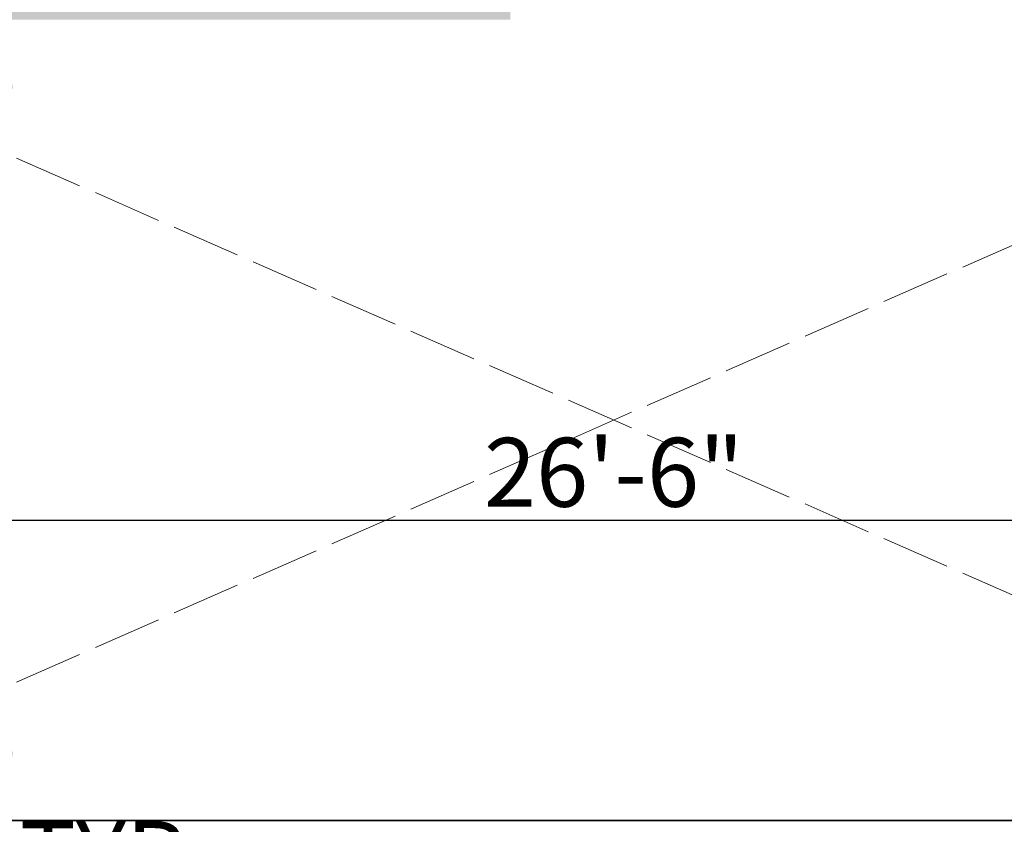
# Model space of a CAD drawing. Units: inches. Extents: x 2083 to 3317, y 1141 to 2115.
# Tile 107 of 256: x 2600 to 2772, y 1272 to 1412. Entities that reach past the tile are written whole.
import ezdxf

# ---------------------------------------------------------------- set-up
doc = ezdxf.new("R2010")
doc.units = ezdxf.units.IN
doc.linetypes.add('ACAD_ISO02W100', pattern=[15, 12, -3])
for name, color, linetype, lineweight in [('A-ANNO-DIMS', 2, 'Continuous', 18), ('A-FLOR-OPEN', 8, 'ACAD_ISO02W100', 13), ('A-WALL', 7, 'Continuous', 35)]:
    doc.layers.add(name, color=color, linetype=linetype, lineweight=lineweight)
doc.layers.add('A-WALL-PATT', color=251, linetype='Continuous', lineweight=13, true_color=0x636466)
doc.styles.get("Standard").update_dxf_attribs({"font": 'arial.ttf'})
doc.dimstyles.new('ISO-25', dxfattribs={"dimtxt": 12, "dimasz": 12, "dimexe": 1.25, "dimexo": 0.625, "dimtad": 1, "dimlunit": 3, "dimtxsty": 'Standard', "dimcen": 2.5, "dimadec": 0, "dimazin": 0, "dimtfac": 1, "dimtmove": 0, "dimatfit": 3, "dimfxl": 1, "dimarcsym": 0})

# ---------------------------------------------------------------- blocks, each defined once
blk = doc.blocks.new('*D25')
at = {"layer": 'A-ANNO-DIMS', "color": 0, "lineweight": -2, "transparency": 16777216}
for p, q in [((2511.96, 1271.64), (2511.96, 1256.61)), ((2535.96, 1271.64), (2535.96, 1256.61)), ((2499.96, 1257.86), (2487.96, 1257.86)), ((2511.96, 1257.86), (2535.96, 1257.86)), ((2547.96, 1257.86), (2634.56, 1257.86))]:
    blk.add_line(p, q, dxfattribs=at)
at = {"layer": 'A-ANNO-DIMS', "color": 0, "transparency": 16777216}
for points in [[(2499.96, 1259.86), (2499.96, 1255.86), (2511.96, 1257.86)], [(2547.96, 1259.86), (2547.96, 1255.86), (2535.96, 1257.86)]]:
    blk.add_solid(points, dxfattribs=at)
at = {"layer": 'Defpoints', "color": 0, "transparency": 16777216}
for p in [(2511.96, 1272.26), (2535.96, 1272.26), (2535.96, 1257.86)]:
    blk.add_point(p, dxfattribs=at)
at = {"layer": 'A-ANNO-DIMS', "color": 0, "transparency": 16777216, "insert": (2597.26, 1264.61), "char_height": 12, "attachment_point": 5}
blk.add_mtext('2\'-0" TYP.', dxfattribs=at)
blk = doc.blocks.new('*D66')
at = {"layer": 'A-ANNO-DIMS', "color": 0, "lineweight": -2, "transparency": 16777216}
for p, q in [((2544.96, 1272.89), (2544.96, 1325.86)), ((2556.96, 1324.61), (2850.96, 1324.61)), ((2862.96, 1272.89), (2862.96, 1325.86))]:
    blk.add_line(p, q, dxfattribs=at)
at = {"layer": 'A-ANNO-DIMS', "color": 0, "transparency": 16777216}
for points in [[(2556.96, 1326.61), (2556.96, 1322.61), (2544.96, 1324.61)], [(2850.96, 1326.61), (2850.96, 1322.61), (2862.96, 1324.61)]]:
    blk.add_solid(points, dxfattribs=at)
at = {"layer": 'Defpoints', "color": 0, "transparency": 16777216}
for p in [(2862.96, 1324.61), (2544.96, 1272.26), (2862.96, 1272.26)]:
    blk.add_point(p, dxfattribs=at)
at = {"layer": 'A-ANNO-DIMS', "color": 0, "transparency": 16777216, "insert": (2703.96, 1331.36), "char_height": 12, "attachment_point": 5}
blk.add_mtext('26\'-6"', dxfattribs=at)
blk = doc.blocks.new('*D67')
at = {"layer": 'A-ANNO-DIMS', "color": 0, "lineweight": -2, "transparency": 16777216}
for p, q in [((2545.58, 1411.76), (2598.56, 1411.76)), ((2597.31, 1399.76), (2597.31, 1284.26)), ((2545.58, 1272.26), (2598.56, 1272.26))]:
    blk.add_line(p, q, dxfattribs=at)
at = {"layer": 'A-ANNO-DIMS', "color": 0, "transparency": 16777216}
for points in [[(2595.31, 1399.76), (2599.31, 1399.76), (2597.31, 1411.76)], [(2595.31, 1284.26), (2599.31, 1284.26), (2597.31, 1272.26)]]:
    blk.add_solid(points, dxfattribs=at)
at = {"layer": 'Defpoints', "color": 0, "transparency": 16777216}
for p in [(2544.96, 1411.76), (2544.96, 1272.26), (2597.31, 1272.26)]:
    blk.add_point(p, dxfattribs=at)
at = {"layer": 'A-ANNO-DIMS', "color": 0, "transparency": 16777216, "insert": (2590.48, 1342.01), "char_height": 12, "attachment_point": 5, "rotation": 90}
blk.add_mtext('11\'-7 1/2"', dxfattribs=at)

msp = doc.modelspace()

# ---------------------------------------------------------------- hatches: boundary and pattern name
at = {"layer": 'A-WALL-PATT'}
h = msp.add_hatch(color=256, dxfattribs=at)
h.dxf.hatch_style = 1
h.paths.add_polyline_path([(3126.96, 2020.761), (2748.96, 2020.761), (2604.96, 2020.761), (2226.96, 2020.761), (2226.96, 1702.761), (2466.96, 1702.761), (2466.96, 1582.761), (2418.96, 1582.761), (2418.96, 1477.761), (2226.96, 1477.761), (2226.96, 1263.261), (2544.96, 1263.261), (2544.96, 1411.761), (2604.96, 1411.761), (2685.96, 1411.761), (2685.96, 1420.761), (2604.96, 1420.761), (2604.96, 1573.761), (2604.96, 1702.761), (2604.96, 2011.761), (2748.96, 2011.761), (2748.96, 1702.761), (2862.96, 1702.761), (2862.96, 1621.761), (2871.96, 1621.761), (2871.96, 1702.761), (2883.96, 1702.761), (2883.96, 1706.939, -0.0264593), (2883.96, 1711.761), (2757.96, 1711.761), (2757.96, 1807.761), (2787.96, 1807.761), (2787.96, 1812.261), (2757.96, 1812.261), (2757.96, 2011.761), (2877.96, 2011.761), (2877.96, 1812.261), (2847.96, 1812.261), (2847.96, 1807.761), (2889.836, 1807.761), (2889.836, 1812.261), (2882.46, 1812.261), (2882.46, 2011.761), (3117.96, 2011.761), (3117.96, 1812.261), (2937.836, 1812.261), (2937.836, 1807.761), (2995.71, 1807.761), (2995.71, 1796.118), (3000.21, 1796.118), (3000.21, 1807.761), (3117.96, 1807.761), (3117.96, 1711.761), (3000.21, 1711.761), (3000.21, 1760.118), (2998.573, 1760.118, -0.020711), (2995.71, 1760.118), (2995.71, 1711.761), (2931.96, 1711.761), (2931.96, 1702.761), (3126.96, 1702.761)])
h.paths.add_polyline_path([(2471.46, 2011.761), (2471.46, 1810.011), (2462.717, 1810.011), (2462.717, 1805.511), (2505.96, 1805.511), (2505.96, 1810.011), (2475.96, 1810.011), (2475.96, 2011.761), (2595.96, 2011.761), (2595.96, 1810.011), (2565.96, 1810.011), (2565.96, 1805.511), (2595.96, 1805.511), (2595.96, 1711.761), (2235.96, 1711.761), (2235.96, 1805.511), (2353.71, 1805.511), (2353.71, 1796.054), (2358.21, 1796.054), (2358.21, 1805.511), (2414.717, 1805.511), (2414.717, 1810.011), (2235.96, 1810.011), (2235.96, 2011.761)], flags=16)
h.paths.add_polyline_path([(2270.205, 1994.61), (2270.205, 1970.61), (2246.205, 1970.61), (2246.205, 1994.61)], flags=0)
edge = h.paths.add_edge_path(flags=0)
edge.add_ellipse((2332.027, 1899.798), major_axis=(-3.043, 3.043), ratio=0.1682525, start_angle=-161.33217, end_angle=-156.30711, ccw=False)
edge.add_ellipse((2333.082, 1898.744), major_axis=(-1.055, 1.055), ratio=0.4535321, start_angle=-123.37102, end_angle=-94.15911)
edge = h.paths.add_edge_path(flags=0)
edge.add_ellipse((2332.027, 1968.876), major_axis=(3.043, 3.043), ratio=0.1682525, start_angle=18.66783, end_angle=23.69289)
edge.add_spline(control_points=[(2332.926, 1970.691), (2332.227, 1970.336), (2330.894, 1969.659), (2328.413, 1970.932), (2327.204, 1967.749), (2324.71, 1969.956), (2322.533, 1967.012), (2320.013, 1971.296), (2317.68, 1968.158), (2316.041, 1967.102), (2315.427, 1966.81)], knot_values=[0, 0, 0, 0, 2.2670587, 4.3245589, 6.6855835, 8.8786411, 11.121502, 14.300359, 17.7552837, 19.732645, 19.732645, 19.732645, 19.732645], degree=3, periodic=0)
edge.add_ellipse((2332.027, 1968.876), major_axis=(3.043, 3.043), ratio=0.1682525, start_angle=18.66783, end_angle=23.69289, ccw=False)
edge.add_ellipse((2333.082, 1969.931), major_axis=(1.055, 1.055), ratio=0.4535321, start_angle=56.62898, end_angle=85.84089, ccw=False)
edge = h.paths.add_edge_path(flags=0)
edge.add_spline(control_points=[(2296.428, 1967.988), (2293.628, 1965.336), (2287.704, 1959.727), (2299.744, 1949.996), (2294.533, 1935.669), (2290.573, 1920.604), (2293.394, 1909.974), (2296.185, 1904.967)], knot_values=[0.0991853, 0.0991853, 0.0991853, 0.0991853, 0.3453009, 0.6198217, 0.9826526, 1.3860932, 1.8105546, 1.8105546, 1.8105546, 1.8105546], degree=3, periodic=0)
edge.add_spline(control_points=[(2296.185, 1904.967), (2297.384, 1902.619), (2298.001, 1901.949), (2298.553, 1901.468)], knot_values=[0.0062457, 0.0062457, 0.0062457, 0.0062457, 0.0554759, 0.0554759, 0.0554759, 0.0554759], degree=3, periodic=0)
edge.add_spline(control_points=[(2298.553, 1901.468), (2297.259, 1900.923), (2295.225, 1900.232), (2293.06, 1900.614), (2292.101, 1900.788), (2292.09, 1900.791)], knot_values=[0.3128349, 0.3128349, 0.3128349, 0.3128349, 0.4017797, 0.4749867, 0.4759027, 0.4759027, 0.4759027, 0.4759027], degree=3, periodic=0)
edge.add_arc((2292.794, 1904.664), 3.937, 215.4209, 259.69818, ccw=False)
edge.add_spline(control_points=[(2289.585, 1902.382), (2289.477, 1902.535), (2289.368, 1902.688), (2289.261, 1902.841)], knot_values=[0.1028719, 0.1028719, 0.1028719, 0.1028719, 0.1168958, 0.1168958, 0.1168958, 0.1168958], degree=3, periodic=0)
edge.add_spline(control_points=[(2289.261, 1902.841), (2288.687, 1902.55), (2287.64, 1902.02), (2285.881, 1901.874), (2283.853, 1901.504), (2281.72, 1899.711), (2278.467, 1899.493), (2276.157, 1901.883), (2272.259, 1899.804), (2267.778, 1901.843), (2262.244, 1900.184), (2257.415, 1901.782), (2254.318, 1900.726), (2253.178, 1900.337)], knot_values=[0, 0, 0, 0, 1.9079767, 3.4771759, 5.261074, 7.9728515, 11.6802485, 13.7179214, 16.9395917, 22.789562, 27.5025027, 33.5952153, 37.1456181, 37.1456181, 37.1456181, 37.1456181], degree=3, periodic=0)
edge.add_line((2253.178, 1900.337), (2250.244, 1902.841))
edge.add_line((2250.244, 1902.841), (2250.244, 1965.833))
edge.add_line((2250.244, 1965.833), (2253.178, 1968.337))
edge.add_spline(control_points=[(2253.178, 1968.337), (2254.318, 1967.948), (2257.415, 1966.892), (2262.244, 1968.49), (2267.778, 1966.831), (2271.527, 1968.537), (2273.876, 1967.828), (2274.207, 1967.728)], knot_values=[0, 0, 0, 0, 0.0901802, 0.2449351, 0.3646438, 0.5132331, 0.5378548, 0.5378548, 0.5378548, 0.5378548], degree=3, periodic=0)
edge.add_arc((2274.353, 1963.793), 3.937, 72.05113, 92.12795, ccw=False)
edge.add_arc((2281.297, 1985.23), 18.596, 252.05113, 288.56572)
edge.add_arc((2292.317, 1956.029), 12.646, 71.02679, 113.77822, ccw=False)
edge = h.paths.add_edge_path(flags=0)
edge.add_spline(control_points=[(2274.899, 1951.856), (2275.066, 1951.617), (2275.233, 1951.377), (2275.398, 1951.136)], knot_values=[1.4099157, 1.4099157, 1.4099157, 1.4099157, 1.4315903, 1.4315903, 1.4315903, 1.4315903], degree=3, periodic=0)
edge.add_spline(control_points=[(2275.398, 1951.136), (2275.792, 1950.562), (2276.179, 1949.984), (2276.546, 1949.397)], knot_values=[1.3582378, 1.3582378, 1.3582378, 1.3582378, 1.4099157, 1.4099157, 1.4099157, 1.4099157], degree=3, periodic=0)
edge.add_line((2276.546, 1949.397), (2277.437, 1947.862))
edge.add_spline(control_points=[(2277.437, 1947.862), (2276.304, 1945.673), (2274.64, 1942.427), (2274.632, 1938.094), (2272.799, 1930.852), (2274.356, 1943.897), (2275.948, 1947.923), (2276.546, 1949.397)], knot_values=[0.0056315, 0.0056315, 0.0056315, 0.0056315, 0.1860139, 0.2660015, 0.3570872, 0.5963902, 0.7397317, 0.7397317, 0.7397317, 0.7397317], degree=3, periodic=0)
edge.add_spline(control_points=[(2276.546, 1949.397), (2276.179, 1949.984), (2275.792, 1950.562), (2275.398, 1951.136)], knot_values=[1.3582378, 1.3582378, 1.3582378, 1.3582378, 1.4099157, 1.4099157, 1.4099157, 1.4099157], degree=3, periodic=0)
edge.add_spline(control_points=[(2275.398, 1951.136), (2274.943, 1950.08), (2274.208, 1948.025), (2273.935, 1944.851), (2272.469, 1937.627), (2273.466, 1945.696), (2274.701, 1951.059), (2274.899, 1951.856)], knot_values=[0.1043639, 0.1043639, 0.1043639, 0.1043639, 0.1896363, 0.2696239, 0.3607096, 0.6000126, 0.6446217, 0.6446217, 0.6446217, 0.6446217], degree=3, periodic=0)
h.paths.add_polyline_path([(2269.168, 1963.128, -0.3575267), (2268.171, 1960.976, -0.0925607), (2268.171, 1939.436, -0.3575267), (2269.168, 1937.285, -0.3575267), (2267.016, 1938.282, -0.1647847), (2254.686, 1938.282, -0.3575267), (2252.534, 1937.285, -0.3575267), (2253.531, 1939.436, -0.0925607), (2253.531, 1960.976, -0.3575267), (2252.534, 1963.128, -0.3575267), (2254.686, 1962.131, -0.1647847), (2267.016, 1962.131, -0.3575267)], flags=0)
h.paths.add_polyline_path([(2248.874, 1967.802), (2248.874, 1957.028), (2249.458, 1957.028), (2249.458, 1911.647), (2248.874, 1911.647), (2248.874, 1900.873), (2246.512, 1900.873, 0.1973271), (2244.15, 1902.457), (2244.15, 1966.218, 0.1973271), (2246.512, 1967.802)], flags=0)
h.paths.add_polyline_path([(2269.168, 1931.389, -0.3575267), (2268.171, 1929.238, -0.0925607), (2268.171, 1907.698, -0.3575267), (2269.168, 1905.547, -0.3575267), (2267.016, 1906.544, -0.1647847), (2254.686, 1906.544, -0.3575267), (2252.534, 1905.547, -0.3575267), (2253.531, 1907.698, -0.0925607), (2253.531, 1929.238, -0.3575267), (2252.534, 1931.389, -0.3575267), (2254.686, 1930.392, -0.1647847), (2267.016, 1930.392, -0.3575267)], flags=0)
edge = h.paths.add_edge_path(flags=0)
edge.add_spline(control_points=[(2276.197, 1906.724), (2276.168, 1909.029), (2276.114, 1913.372), (2270.598, 1924.925), (2273.905, 1919.013), (2275.922, 1916.262), (2275.475, 1912.402), (2277.258, 1910.381), (2276.696, 1908.225), (2276.646, 1906.813), (2276.618, 1906.008)], knot_values=[0, 0, 0, 0, 8.6102597, 16.2212739, 18.8430575, 23.8048978, 27.4408283, 29.3561016, 31.2034776, 33.6506866, 33.6506866, 33.6506866, 33.6506866], degree=3, periodic=0)
edge.add_spline(control_points=[(2276.618, 1906.008), (2276.623, 1905.624), (2276.498, 1904.629), (2275.442, 1903.855), (2274.937, 1903.08), (2274.859, 1902.841)], knot_values=[0.1564884, 0.1564884, 0.1564884, 0.1564884, 0.1843975, 0.2313765, 0.2505985, 0.2505985, 0.2505985, 0.2505985], degree=3, periodic=0)
edge.add_line((2274.859, 1902.841), (2276.506, 1902.841))
edge.add_spline(control_points=[(2276.506, 1902.841), (2276.788, 1903.085), (2277.665, 1904.125), (2278.25, 1904.341), (2277.654, 1908.527), (2278.156, 1906.228), (2278.1, 1905.286), (2278.847, 1904.069), (2277.857, 1903.415), (2277.874, 1902.991), (2277.904, 1902.841)], knot_values=[0.0595743, 0.0595743, 0.0595743, 0.0595743, 0.0807529, 0.1037415, 0.1697201, 0.1760361, 0.2071372, 0.2404744, 0.2623409, 0.2736605, 0.2736605, 0.2736605, 0.2736605], degree=3, periodic=0)
edge.add_line((2277.904, 1902.841), (2280.03, 1902.841))
edge.add_spline(control_points=[(2280.03, 1902.841), (2279.888, 1903.088), (2279.499, 1903.982), (2280.152, 1905.939), (2278.104, 1909.658), (2279.762, 1907.185), (2280.328, 1904.875), (2280.485, 1903.49), (2281.463, 1903.249), (2281.758, 1902.936), (2281.834, 1902.841)], knot_values=[0.013856, 0.013856, 0.013856, 0.013856, 0.0348738, 0.0888667, 0.1078792, 0.1267378, 0.158714, 0.1937575, 0.2174868, 0.2267221, 0.2267221, 0.2267221, 0.2267221], degree=3, periodic=0)
edge.add_spline(control_points=[(2281.834, 1902.841), (2281.788, 1902.827), (2281.647, 1902.783), (2281.396, 1902.859), (2281.088, 1902.985), (2280.721, 1903.061), (2280.333, 1903.026), (2280.125, 1902.899), (2280.03, 1902.841)], knot_values=[0, 0, 0, 0, 0.1441304, 0.435517, 0.7492759, 1.1530457, 1.5483707, 1.878348, 1.878348, 1.878348, 1.878348], degree=3, periodic=0)
edge.add_line((2280.03, 1902.841), (2277.904, 1902.841))
edge.add_spline(control_points=[(2277.904, 1902.841), (2277.893, 1902.796), (2277.865, 1902.68), (2277.607, 1902.687), (2277.274, 1902.801), (2276.838, 1902.62), (2276.584, 1902.789), (2276.506, 1902.841)], knot_values=[0, 0, 0, 0, 0.1271885, 0.3261988, 0.6280094, 1.2435704, 1.5153306, 1.5153306, 1.5153306, 1.5153306], degree=3, periodic=0)
edge.add_line((2276.506, 1902.841), (2274.859, 1902.841))
edge.add_spline(control_points=[(2274.859, 1902.841), (2274.814, 1902.899), (2274.725, 1903.013), (2274.493, 1903.119), (2274.244, 1902.961), (2273.937, 1903.185), (2273.614, 1902.983), (2273.408, 1902.883), (2273.322, 1902.841)], knot_values=[0, 0, 0, 0, 0.2184302, 0.4369566, 0.6879766, 0.9903786, 1.3983955, 1.6918498, 1.6918498, 1.6918498, 1.6918498], degree=3, periodic=0)
edge.add_spline(control_points=[(2273.322, 1902.841), (2273.617, 1903.446), (2274.274, 1904.538), (2276.027, 1904.574), (2276.207, 1906.584), (2276.197, 1906.724)], knot_values=[0.0122268, 0.0122268, 0.0122268, 0.0122268, 0.0594721, 0.1062177, 0.134458, 0.134458, 0.134458, 0.134458], degree=3, periodic=0)
h.paths.add_polyline_path([(2270.776, 1897.79), (2270.776, 1873.79), (2246.776, 1873.79), (2246.776, 1897.79)], flags=0)
h.paths.add_polyline_path([(2353.71, 1760.005), (2353.71, 1760.054), (2358.21, 1760.054, -0.033729)], flags=0)
h.paths.add_polyline_path([(2321.819, 1737.529), (2341.995, 1737.529, -0.4142136), (2343.203, 1736.321), (2343.203, 1721.021, -0.4142136), (2341.995, 1719.813), (2321.819, 1719.813, -0.4142136), (2320.611, 1721.021), (2320.611, 1736.321, -0.4142136)], flags=0)
h.paths.add_polyline_path([(2324.235, 1736.321), (2339.579, 1736.321, -0.4142136), (2341.995, 1733.905), (2341.995, 1725.45, -0.4142136), (2339.579, 1723.034), (2333.681, 1723.034), (2333.845, 1722.045, -0.8706461), (2335.425, 1721.826, -0.767327), (2333.923, 1721.423), (2331.291, 1721.423, -0.767327), (2329.788, 1721.826, -0.8706461), (2331.368, 1722.045), (2331.533, 1723.034), (2324.235, 1723.034, -0.4142136), (2321.819, 1725.45), (2321.819, 1733.905, -0.4142136)], flags=0)
h.paths.add_polyline_path([(2570.484, 1928.615), (2589.684, 1928.615), (2590.169, 1928.615), (2590.169, 1904.993), (2570.484, 1904.993)], flags=0)
h.paths.add_polyline_path([(2574.447, 1927.264, -1), (2572.829, 1927.264, -1)], flags=0)
h.paths.add_polyline_path([(2573.09, 1926.941), (2573.925, 1927.776), (2574.148, 1927.553), (2573.313, 1926.718)], flags=0)
h.paths.add_polyline_path([(2578.779, 1919.73, -1), (2571.592, 1919.73, -1)], flags=0)
h.paths.add_polyline_path([(2578.385, 1919.73, -1), (2571.985, 1919.73, -1)], flags=0)
h.paths.add_polyline_path([(2331.596, 1729.476, -1), (2333.618, 1729.476, -1)], flags=0)
h.paths.add_polyline_path([(2578.034, 1927.264, -1), (2576.416, 1927.264, -1)], flags=0)
h.paths.add_polyline_path([(2576.689, 1927.531), (2576.912, 1927.754), (2577.747, 1926.919), (2577.524, 1926.696)], flags=0)
h.paths.add_polyline_path([(2578.139, 1909.86, -1), (2572.232, 1909.86, -1)], flags=0)
h.paths.add_polyline_path([(2577.745, 1909.86, -1), (2572.625, 1909.86, -1)], flags=0)
h.paths.add_polyline_path([(2583.798, 1927.264, -1), (2582.179, 1927.264, -1)], flags=0)
h.paths.add_polyline_path([(2582.719, 1927.754), (2583.554, 1926.919), (2583.331, 1926.696), (2582.496, 1927.531)], flags=0)
h.paths.add_polyline_path([(2582.496, 1927.531), (2582.719, 1927.754), (2583.554, 1926.919), (2583.331, 1926.696)], flags=0)
h.paths.add_polyline_path([(2587.739, 1920.53, -1), (2581.832, 1920.53, -1)], flags=0)
h.paths.add_polyline_path([(2587.345, 1920.53, -1), (2582.225, 1920.53, -1)], flags=0)
h.paths.add_polyline_path([(2587.385, 1927.264, -1), (2585.766, 1927.264, -1)], flags=0)
h.paths.add_polyline_path([(2586.082, 1926.98), (2586.917, 1927.815), (2587.14, 1927.593), (2586.305, 1926.758)], flags=0)
h.paths.add_polyline_path([(2588.379, 1910.66, -1), (2581.192, 1910.66, -1)], flags=0)
h.paths.add_polyline_path([(2587.985, 1910.66, -1), (2581.585, 1910.66, -1)], flags=0)
h.paths.add_polyline_path([(2417.168, 1729.478), (2437.344, 1729.478, -0.4142136), (2438.552, 1728.27), (2438.552, 1712.969, -0.4142136), (2437.344, 1711.761), (2417.168, 1711.761, -0.4142136), (2415.96, 1712.969), (2415.96, 1728.27, -0.4142136)], flags=0)
h.paths.add_polyline_path([(2419.584, 1728.27), (2434.928, 1728.27, -0.4142136), (2437.344, 1725.854), (2437.344, 1717.398, -0.4142136), (2434.928, 1714.983), (2429.029, 1714.983), (2429.194, 1713.994, -0.8706461), (2430.774, 1713.775, -0.767327), (2429.271, 1713.372), (2426.64, 1713.372, -0.767327), (2425.137, 1713.775, -0.8706461), (2426.717, 1713.994), (2426.882, 1714.983), (2419.584, 1714.983, -0.4142136), (2417.168, 1717.398), (2417.168, 1725.854, -0.4142136)], flags=0)
h.paths.add_polyline_path([(2419.584, 1728.27), (2434.928, 1728.27, -0.4142136), (2437.344, 1725.854), (2437.344, 1717.398, -0.4142136), (2434.928, 1714.983), (2429.029, 1714.983), (2428.358, 1719.009), (2427.553, 1719.009), (2426.882, 1714.983), (2419.584, 1714.983, -0.4142136), (2417.168, 1717.398), (2417.168, 1725.854, -0.4142136)], flags=0)
h.paths.add_polyline_path([(2426.944, 1721.425, -1), (2428.967, 1721.425, -1)], flags=0)
h.paths.add_polyline_path([(2475.96, 1702.761), (2595.96, 1702.761), (2595.96, 1582.761), (2475.96, 1582.761)], flags=16)
h.paths.add_polyline_path([(2427.96, 1573.761), (2595.96, 1573.761), (2595.96, 1468.761), (2595.96, 1420.761), (2384.46, 1420.761), (2384.46, 1468.761), (2427.96, 1468.761)], flags=16)
h.paths.add_polyline_path([(2379.96, 1468.761), (2379.96, 1420.761), (2235.96, 1420.761), (2235.96, 1468.761)], flags=16)
h.paths.add_polyline_path([(2317.816, 1466.696), (2337.992, 1466.696, -0.4142136), (2339.2, 1465.488), (2339.2, 1450.187, -0.4142136), (2337.992, 1448.979), (2317.816, 1448.979, -0.4142136), (2316.608, 1450.187), (2316.608, 1465.488, -0.4142136)], flags=0)
h.paths.add_polyline_path([(2320.232, 1465.488), (2335.576, 1465.488, -0.4142136), (2337.992, 1463.072), (2337.992, 1454.616, -0.4142136), (2335.576, 1452.2), (2329.677, 1452.2), (2329.842, 1451.212, -0.8706461), (2331.422, 1450.992, -0.767327), (2329.92, 1450.59), (2327.288, 1450.59, -0.767327), (2325.785, 1450.992, -0.8706461), (2327.365, 1451.212), (2327.53, 1452.2), (2320.232, 1452.2, -0.4142136), (2317.816, 1454.616), (2317.816, 1463.072, -0.4142136)], flags=0)
h.paths.add_polyline_path([(2320.232, 1465.488), (2335.576, 1465.488, -0.4142136), (2337.992, 1463.072), (2337.992, 1454.616, -0.4142136), (2335.576, 1452.2), (2329.677, 1452.2), (2329.006, 1456.227), (2328.201, 1456.227), (2327.53, 1452.2), (2320.232, 1452.2, -0.4142136), (2317.816, 1454.616), (2317.816, 1463.072, -0.4142136)], flags=0)
h.paths.add_polyline_path([(2327.593, 1458.643, -1), (2329.615, 1458.643, -1)], flags=0)
h.paths.add_polyline_path([(2244.412, 1433.34), (2241.921, 1433.34, -0.4142136), (2240.018, 1435.244), (2240.018, 1440.953, -0.4142105), (2241.921, 1442.856), (2244.412, 1442.856, -1.9764724)], flags=0)
h.paths.add_polyline_path([(2245.357, 1434.398, -0.4142136), (2245.357, 1441.799, -2.1440985)], flags=0)
h.paths.add_polyline_path([(2535.96, 1416.261), (2535.96, 1272.261), (2235.96, 1272.261), (2235.96, 1416.261)], flags=16)
h.paths.add_polyline_path([(2260.12, 1384.293), (2260.12, 1362.039), (2237.865, 1362.039), (2237.865, 1384.293)], flags=0)
edge = h.paths.add_edge_path(flags=0)
edge.add_line((2318.252, 1362.093), (2318.146, 1362.001))
edge.add_ellipse((2317.445, 1360.431), major_axis=(2.822, 2.822), ratio=0.1682525, start_angle=18.66783, end_angle=20.94813, ccw=False)
edge.add_ellipse((2318.423, 1361.409), major_axis=(0.978, 0.978), ratio=0.4535321, start_angle=56.62898, end_angle=70.2262, ccw=False)
edge = h.paths.add_edge_path(flags=0)
edge.add_line((2319.107, 1295.571), (2319.015, 1295.677))
edge.add_ellipse((2317.445, 1296.378), major_axis=(-2.822, 2.822), ratio=0.1682525, start_angle=-161.33217, end_angle=-159.05187, ccw=False)
edge.add_ellipse((2318.423, 1295.4), major_axis=(-0.978, 0.978), ratio=0.4535321, start_angle=-123.37102, end_angle=-109.7738)
edge = h.paths.add_edge_path(flags=0)
edge.add_spline(control_points=[(2284.21, 1301.17), (2284.581, 1300.445), (2284.891, 1299.892), (2285.16, 1299.461)], knot_values=[0.0390658, 0.0390658, 0.0390658, 0.0390658, 0.0554759, 0.0554759, 0.0554759, 0.0554759], degree=3, periodic=0)
edge.add_line((2285.16, 1299.461), (2284.21, 1301.17))
edge = h.paths.add_edge_path(flags=0)
edge.add_line((2280.412, 1297.298), (2283.37, 1297.036))
edge.add_line((2283.37, 1297.036), (2286.406, 1297.926))
edge.add_spline(control_points=[(2286.406, 1297.926), (2285.305, 1297.463), (2284.345, 1297.129), (2283.37, 1297.036)], knot_values=[0.3943688, 0.3943688, 0.3943688, 0.3943688, 0.4759027, 0.4759027, 0.4759027, 0.4759027], degree=3, periodic=0)
edge.add_spline(control_points=[(2283.37, 1297.036), (2283.281, 1297.028), (2282.316, 1296.957), (2281.313, 1297.134), (2280.423, 1297.296), (2280.412, 1297.298)], knot_values=[0.3128349, 0.3128349, 0.3128349, 0.3128349, 0.3202458, 0.3934528, 0.3943688, 0.3943688, 0.3943688, 0.3943688], degree=3, periodic=0)
edge = h.paths.add_edge_path(flags=0)
edge.add_line((2284.436, 1359.607), (2280.446, 1355.328))
edge.add_line((2280.446, 1355.328), (2279.58, 1351.018))
edge.add_line((2279.58, 1351.018), (2282.413, 1346.58))
edge.add_spline(control_points=[(2282.413, 1346.58), (2283.153, 1345.589), (2284.253, 1344.029), (2284.801, 1342.387), (2284.935, 1341.806)], knot_values=[1.2400982, 1.2400982, 1.2400982, 1.2400982, 1.3328922, 1.3827123, 1.3827123, 1.3827123, 1.3827123], degree=3, periodic=0)
edge.add_spline(control_points=[(2284.935, 1341.806), (2285.319, 1340.141), (2285.233, 1338.409), (2284.91, 1336.654)], knot_values=[1.0974841, 1.0974841, 1.0974841, 1.0974841, 1.2400982, 1.2400982, 1.2400982, 1.2400982], degree=3, periodic=0)
edge.add_spline(control_points=[(2284.91, 1336.654), (2284.587, 1334.899), (2284.027, 1333.12), (2283.463, 1331.361)], knot_values=[0.9548699, 0.9548699, 0.9548699, 0.9548699, 1.0974841, 1.0974841, 1.0974841, 1.0974841], degree=3, periodic=0)
edge.add_line((2283.463, 1331.361), (2281.89, 1326.153))
edge.add_line((2281.89, 1326.153), (2280.756, 1321.056))
edge.add_line((2280.756, 1321.056), (2280.299, 1316.002))
edge.add_line((2280.299, 1316.002), (2280.716, 1310.95))
edge.add_line((2280.716, 1310.95), (2282.028, 1305.972))
edge.add_line((2282.028, 1305.972), (2284.21, 1301.17))
edge.add_spline(control_points=[(2284.21, 1301.17), (2283.341, 1302.73), (2282.612, 1304.336), (2282.028, 1305.972)], knot_values=[0.0991853, 0.0991853, 0.0991853, 0.0991853, 0.2417994, 0.2417994, 0.2417994, 0.2417994], degree=3, periodic=0)
edge.add_spline(control_points=[(2282.028, 1305.972), (2281.444, 1307.608), (2281.005, 1309.273), (2280.716, 1310.95)], knot_values=[0.2417994, 0.2417994, 0.2417994, 0.2417994, 0.3844135, 0.3844135, 0.3844135, 0.3844135], degree=3, periodic=0)
edge.add_spline(control_points=[(2280.716, 1310.95), (2280.433, 1312.588), (2280.289, 1314.277), (2280.299, 1315.962), (2280.299, 1316.002)], knot_values=[0.3844135, 0.3844135, 0.3844135, 0.3844135, 0.5236467, 0.5270276, 0.5270276, 0.5270276, 0.5270276], degree=3, periodic=0)
edge.add_spline(control_points=[(2280.299, 1316.002), (2280.312, 1317.687), (2280.478, 1319.368), (2280.756, 1321.056)], knot_values=[0.5270276, 0.5270276, 0.5270276, 0.5270276, 0.6696417, 0.6696417, 0.6696417, 0.6696417], degree=3, periodic=0)
edge.add_spline(control_points=[(2280.756, 1321.056), (2281.035, 1322.744), (2281.426, 1324.44), (2281.89, 1326.153)], knot_values=[0.6696417, 0.6696417, 0.6696417, 0.6696417, 0.8122558, 0.8122558, 0.8122558, 0.8122558], degree=3, periodic=0)
edge.add_spline(control_points=[(2281.89, 1326.153), (2282.264, 1327.533), (2282.788, 1329.262), (2283.353, 1331.018), (2283.463, 1331.361)], knot_values=[0.8122558, 0.8122558, 0.8122558, 0.8122558, 0.9270873, 0.9548699, 0.9548699, 0.9548699, 0.9548699], degree=3, periodic=0)
edge.add_line((2283.463, 1331.361), (2284.91, 1336.654))
edge.add_line((2284.91, 1336.654), (2284.935, 1341.806))
edge.add_line((2284.935, 1341.806), (2282.413, 1346.58))
edge.add_spline(control_points=[(2282.413, 1346.58), (2281.275, 1348.104), (2280.078, 1349.57), (2279.58, 1351.018)], knot_values=[1.3827123, 1.3827123, 1.3827123, 1.3827123, 1.5253264, 1.5253264, 1.5253264, 1.5253264], degree=3, periodic=0)
edge.add_spline(control_points=[(2279.58, 1351.018), (2279.443, 1351.415), (2279.136, 1352.857), (2279.735, 1354.29), (2280.446, 1355.328)], knot_values=[1.5253264, 1.5253264, 1.5253264, 1.5253264, 1.564439, 1.6679405, 1.6679405, 1.6679405, 1.6679405], degree=3, periodic=0)
edge.add_spline(control_points=[(2280.446, 1355.328), (2281.426, 1356.758), (2282.931, 1358.183), (2284.436, 1359.607)], knot_values=[1.6679405, 1.6679405, 1.6679405, 1.6679405, 1.8105546, 1.8105546, 1.8105546, 1.8105546], degree=3, periodic=0)
edge.add_arc((2280.623, 1348.518), 11.726, 71.02679, 113.77822)
edge.add_arc((2270.405, 1375.595), 17.244, 252.05113, 288.56572, ccw=False)
edge.add_arc((2263.966, 1355.718), 3.651, 72.05113, 92.12795)
edge.add_arc((2263.966, 1355.718), 3.651, 92.12795, 177.98513)
edge.add_spline(control_points=[(2260.318, 1355.846), (2260.26, 1354.221), (2260.551, 1350.187), (2262.999, 1346.766), (2264.473, 1344.649)], knot_values=[1.4315903, 1.4315903, 1.4315903, 1.4315903, 1.5641438, 1.7706953, 1.7706953, 1.7706953, 1.7706953], degree=3, periodic=0)
edge.add_line((2264.473, 1344.649), (2264.936, 1343.983))
edge.add_spline(control_points=[(2263.801, 1340.248), (2263.843, 1340.514), (2264.067, 1341.756), (2264.513, 1343.002), (2264.935, 1343.981)], knot_values=[0.5365702, 0.5365702, 0.5365702, 0.5365702, 0.5593494, 0.6446217, 0.6446217, 0.6446217, 0.6446217], degree=3, periodic=0)
edge.add_spline(control_points=[(2264.935, 1343.981), (2265.118, 1343.715), (2265.299, 1343.448), (2265.477, 1343.179)], knot_values=[1.3840767, 1.3840767, 1.3840767, 1.3840767, 1.4099157, 1.4099157, 1.4099157, 1.4099157], degree=3, periodic=0)
edge.add_spline(control_points=[(2265.477, 1343.179), (2265.655, 1342.911), (2265.829, 1342.641), (2265.999, 1342.369)], knot_values=[1.3582378, 1.3582378, 1.3582378, 1.3582378, 1.3840767, 1.3840767, 1.3840767, 1.3840767], degree=3, periodic=0)
edge.add_line((2265.999, 1342.369), (2266.826, 1340.946))
edge.add_spline(control_points=[(2266.826, 1340.946), (2268.894, 1337.09), (2271.398, 1325.843), (2270.516, 1310.569), (2275.919, 1301.861), (2277.79, 1299.199)], knot_values=[0.1168958, 0.1168958, 0.1168958, 0.1168958, 0.4729873, 1.0509689, 1.3137934, 1.3137934, 1.3137934, 1.3137934], degree=3, periodic=0)
edge.add_spline(control_points=[(2277.79, 1299.199), (2277.839, 1299.128), (2277.889, 1299.057), (2277.94, 1298.987)], knot_values=[0.1098839, 0.1098839, 0.1098839, 0.1098839, 0.1168958, 0.1168958, 0.1168958, 0.1168958], degree=3, periodic=0)
edge.add_line((2277.94, 1298.987), (2277.789, 1299.199))
edge.add_spline(control_points=[(2277.789, 1299.199), (2277.257, 1298.929), (2276.286, 1298.438), (2275.039, 1298.334), (2274.383, 1298.239), (2274.215, 1298.209)], knot_values=[33.1218702, 33.1218702, 33.1218702, 33.1218702, 35.0290557, 36.5982549, 37.1448269, 37.1448269, 37.1448269, 37.1448269], degree=3, periodic=0)
edge.add_line((2274.215, 1298.209), (2273.073, 1297.893))
edge.add_spline(control_points=[(2273.073, 1297.893), (2272.323, 1297.58), (2271.039, 1296.511), (2269.248, 1296.226), (2268.423, 1296.375)], knot_values=[26.5325843, 26.5325843, 26.5325843, 26.5325843, 29.198919, 31.8391012, 31.8391012, 31.8391012, 31.8391012], degree=3, periodic=0)
edge.add_line((2268.423, 1296.375), (2263.879, 1297.458))
edge.add_spline(control_points=[(2263.879, 1297.458), (2263.556, 1297.359), (2261.86, 1296.839), (2260.239, 1297.282), (2258.933, 1297.516)], knot_values=[15.9195506, 15.9195506, 15.9195506, 15.9195506, 16.9395917, 21.2260675, 21.2260675, 21.2260675, 21.2260675], degree=3, periodic=0)
edge.add_line((2258.933, 1297.516), (2254.055, 1297.329))
edge.add_spline(control_points=[(2254.055, 1297.329), (2253.756, 1297.296), (2252.114, 1297.165), (2250.462, 1297.544), (2249.13, 1297.668)], knot_values=[5.3065169, 5.3065169, 5.3065169, 5.3065169, 6.2764352, 10.6130337, 10.6130337, 10.6130337, 10.6130337], degree=3, periodic=0)
edge.add_line((2249.13, 1297.668), (2244.332, 1296.878))
edge.add_line((2244.332, 1296.878), (2241.611, 1299.199))
edge.add_line((2241.611, 1299.199), (2241.611, 1357.609))
edge.add_line((2241.611, 1357.609), (2244.332, 1359.931))
edge.add_line((2244.332, 1359.931), (2252.729, 1359.543))
edge.add_spline(control_points=[(2252.729, 1359.543), (2252.871, 1359.546), (2253.306, 1359.548), (2253.74, 1359.514), (2254.032, 1359.482)], knot_values=[0.233291, 0.233291, 0.233291, 0.233291, 0.2449351, 0.2689274, 0.2689274, 0.2689274, 0.2689274], degree=3, periodic=0)
edge.add_line((2254.032, 1359.482), (2259.587, 1359.416))
edge.add_spline(control_points=[(2259.587, 1359.416), (2260.677, 1359.629), (2262.073, 1359.897), (2263.524, 1359.459), (2263.83, 1359.366)], knot_values=[0.4225164, 0.4225164, 0.4225164, 0.4225164, 0.5132331, 0.5378548, 0.5378548, 0.5378548, 0.5378548], degree=3, periodic=0)
edge.add_arc((2263.966, 1355.718), 3.651, 72.05113, 92.12795, ccw=False)
edge.add_arc((2270.405, 1375.595), 17.244, 252.05113, 288.56572)
edge.add_arc((2280.623, 1348.518), 11.726, 71.02679, 113.77822, ccw=False)
h.paths.add_polyline_path([(2240.341, 1359.435), (2240.341, 1349.444), (2240.882, 1349.444), (2240.882, 1307.365), (2240.341, 1307.365), (2240.341, 1297.374), (2238.15, 1297.374, 0.1973271), (2235.96, 1298.843), (2235.96, 1357.966, 0.1973271), (2238.15, 1359.435)], flags=0)
h.paths.add_polyline_path([(2259.158, 1355.101, -0.3575267), (2258.233, 1353.106, -0.0925607), (2258.233, 1333.133, -0.3575267), (2259.158, 1331.138, -0.3575267), (2257.163, 1332.062, -0.1647847), (2245.729, 1332.062, -0.3575267), (2243.735, 1331.138, -0.3575267), (2244.659, 1333.133, -0.0925607), (2244.659, 1353.106, -0.3575267), (2243.735, 1355.101, -0.3575267), (2245.729, 1354.176, -0.1647847), (2257.163, 1354.176, -0.3575267)], flags=0)
edge = h.paths.add_edge_path(flags=0)
edge.add_line((2265.999, 1342.369), (2266.826, 1340.946))
edge.add_line((2266.826, 1340.946), (2265.308, 1337.814))
edge.add_line((2265.308, 1337.814), (2264.358, 1334.653))
edge.add_line((2264.358, 1334.653), (2264.262, 1333.8))
edge.add_spline(control_points=[(2264.262, 1333.8), (2264.208, 1333.187), (2264.162, 1332.366), (2264.007, 1331.414), (2263.969, 1331.202)], knot_values=[0.4644442, 0.4644442, 0.4644442, 0.4644442, 0.5166905, 0.5316081, 0.5316081, 0.5316081, 0.5316081], degree=3, periodic=0)
edge.add_spline(control_points=[(2263.969, 1331.202), (2263.775, 1330.119), (2263.424, 1328.791), (2263.257, 1328.531), (2263.234, 1328.515)], knot_values=[0.3726816, 0.3726816, 0.3726816, 0.3726816, 0.4488497, 0.4644442, 0.4644442, 0.4644442, 0.4644442], degree=3, periodic=0)
edge.add_spline(control_points=[(2263.234, 1328.515), (2263.096, 1328.42), (2263.131, 1329.301), (2263.275, 1330.616)], knot_values=[0.2809191, 0.2809191, 0.2809191, 0.2809191, 0.3726816, 0.3726816, 0.3726816, 0.3726816], degree=3, periodic=0)
edge.add_spline(control_points=[(2263.275, 1330.616), (2263.419, 1331.93), (2263.672, 1333.677), (2263.97, 1335.315)], knot_values=[0.1891566, 0.1891566, 0.1891566, 0.1891566, 0.2809191, 0.2809191, 0.2809191, 0.2809191], degree=3, periodic=0)
edge.add_spline(control_points=[(2263.97, 1335.315), (2264.1, 1336.032), (2264.419, 1337.622), (2264.755, 1338.864), (2264.947, 1339.491)], knot_values=[0.097394, 0.097394, 0.097394, 0.097394, 0.1375775, 0.1891566, 0.1891566, 0.1891566, 0.1891566], degree=3, periodic=0)
edge.add_spline(control_points=[(2264.947, 1339.491), (2265.29, 1340.606), (2265.644, 1341.494), (2265.999, 1342.369)], knot_values=[0.0056315, 0.0056315, 0.0056315, 0.0056315, 0.097394, 0.097394, 0.097394, 0.097394], degree=3, periodic=0)
h.paths.add_polyline_path([(2259.158, 1325.671, -0.3575267), (2258.233, 1323.676, -0.0925607), (2258.233, 1303.703, -0.3575267), (2259.158, 1301.708, -0.3575267), (2257.163, 1302.633, -0.1647847), (2245.729, 1302.633, -0.3575267), (2243.735, 1301.708, -0.3575267), (2244.659, 1303.703, -0.0925607), (2244.659, 1323.676, -0.3575267), (2243.735, 1325.671, -0.3575267), (2245.729, 1324.747, -0.1647847), (2257.163, 1324.747, -0.3575267)], flags=0)
edge = h.paths.add_edge_path(flags=0)
edge.add_spline(control_points=[(2261.709, 1317.311), (2261.679, 1317.418), (2261.762, 1317.389), (2262.491, 1316.09), (2262.962, 1315.301)], knot_values=[14.9558607, 14.9558607, 14.9558607, 14.9558607, 16.2212739, 18.6948259, 18.6948259, 18.6948259, 18.6948259], degree=3, periodic=0)
edge.add_spline(control_points=[(2262.962, 1315.301), (2262.99, 1315.254), (2263.702, 1314.067), (2264.349, 1313.127), (2264.73, 1312.164)], knot_values=[18.6948259, 18.6948259, 18.6948259, 18.6948259, 18.8430575, 22.433791, 22.433791, 22.433791, 22.433791], degree=3, periodic=0)
edge.add_spline(control_points=[(2264.73, 1312.164), (2264.876, 1311.796), (2265.177, 1310.77), (2265.143, 1309.559), (2265.248, 1308.824)], knot_values=[22.433791, 22.433791, 22.433791, 22.433791, 23.8048978, 26.1727562, 26.1727562, 26.1727562, 26.1727562], degree=3, periodic=0)
edge.add_line((2265.248, 1308.824), (2265.851, 1307.172))
edge.add_spline(control_points=[(2265.851, 1307.172), (2266.065, 1306.822), (2266.384, 1306.332), (2266.424, 1305.781), (2266.42, 1305.611)], knot_values=[28.0625624, 28.0625624, 28.0625624, 28.0625624, 29.3561016, 29.9117214, 29.9117214, 29.9117214, 29.9117214], degree=3, periodic=0)
edge.add_spline(control_points=[(2266.42, 1305.611), (2266.416, 1305.433), (2266.394, 1305.25), (2266.365, 1305.066)], knot_values=[29.9117214, 29.9117214, 29.9117214, 29.9117214, 30.4978371, 30.4978371, 30.4978371, 30.4978371], degree=3, periodic=0)
edge.add_line((2266.365, 1305.066), (2266.066, 1302.136))
edge.add_spline(control_points=[(2266.066, 1302.136), (2266.071, 1301.78), (2265.998, 1301.2), (2265.663, 1300.759), (2265.509, 1300.586)], knot_values=[0.1564884, 0.1564884, 0.1564884, 0.1564884, 0.1843975, 0.2035434, 0.2035434, 0.2035434, 0.2035434], degree=3, periodic=0)
edge.add_line((2265.509, 1300.586), (2264.435, 1299.199))
edge.add_line((2264.435, 1299.199), (2265.962, 1299.199))
edge.add_line((2265.962, 1299.199), (2267.336, 1301.175))
edge.add_line((2267.336, 1301.175), (2267.312, 1301.986))
edge.add_spline(control_points=[(2267.312, 1301.986), (2267.261, 1302.862), (2267.16, 1303.737), (2267.271, 1303.326)], knot_values=[0.1262286, 0.1262286, 0.1262286, 0.1262286, 0.1666174, 0.1666174, 0.1666174, 0.1666174], degree=3, periodic=0)
edge.add_spline(control_points=[(2267.271, 1303.326), (2267.28, 1303.294), (2267.31, 1303.175), (2267.373, 1302.884), (2267.406, 1302.683), (2267.418, 1302.601)], knot_values=[0.1666174, 0.1666174, 0.1666174, 0.1666174, 0.1697201, 0.1760361, 0.1807647, 0.1807647, 0.1807647, 0.1807647], degree=3, periodic=0)
edge.add_spline(control_points=[(2267.744, 1300.988), (2267.688, 1301.151), (2267.481, 1301.657), (2267.484, 1302.145), (2267.418, 1302.601)], knot_values=[0.1807647, 0.1807647, 0.1807647, 0.1807647, 0.1937665, 0.2201389, 0.2201389, 0.2201389, 0.2201389], degree=3, periodic=0)
edge.add_line((2267.418, 1302.601), (2267.744, 1300.988))
edge.add_spline(control_points=[(2267.744, 1300.988), (2267.832, 1300.732), (2267.932, 1300.31), (2267.555, 1299.975), (2267.429, 1299.829)], knot_values=[0.2201389, 0.2201389, 0.2201389, 0.2201389, 0.2404744, 0.2548903, 0.2548903, 0.2548903, 0.2548903], degree=3, periodic=0)
edge.add_line((2267.429, 1299.829), (2267.258, 1299.199))
edge.add_line((2267.258, 1299.199), (2269.23, 1299.199))
edge.add_spline(control_points=[(2269.23, 1299.199), (2269.099, 1299.429), (2268.843, 1300.016), (2269.012, 1300.916), (2268.947, 1301.661)], knot_values=[0.013856, 0.013856, 0.013856, 0.013856, 0.0348738, 0.0670726, 0.0670726, 0.0670726, 0.0670726], degree=3, periodic=0)
edge.add_line((2268.947, 1301.661), (2268.432, 1303.603))
edge.add_spline(control_points=[(2268.432, 1303.603), (2268.176, 1304.192), (2267.596, 1305.251), (2268.041, 1304.623), (2268.251, 1304.282)], knot_values=[0.0901547, 0.0901547, 0.0901547, 0.0901547, 0.1078792, 0.1202891, 0.1202891, 0.1202891, 0.1202891], degree=3, periodic=0)
edge.add_spline(control_points=[(2268.251, 1304.282), (2268.361, 1304.105), (2269.058, 1302.918), (2269.383, 1301.59), (2269.521, 1300.776), (2269.575, 1300.556)], knot_values=[0.1202891, 0.1202891, 0.1202891, 0.1202891, 0.1267378, 0.158714, 0.1735056, 0.1735056, 0.1735056, 0.1735056], degree=3, periodic=0)
edge.add_line((2269.575, 1300.556), (2270.686, 1299.421))
edge.add_spline(control_points=[(2270.686, 1299.421), (2270.767, 1299.357), (2270.838, 1299.281), (2270.903, 1299.199)], knot_values=[0.2181597, 0.2181597, 0.2181597, 0.2181597, 0.2267221, 0.2267221, 0.2267221, 0.2267221], degree=3, periodic=0)
edge.add_line((2270.937, 1299.193), (2270.903, 1299.199))
edge.add_spline(control_points=[(2270.903, 1299.199), (2270.86, 1299.186), (2270.73, 1299.146), (2270.496, 1299.216), (2270.272, 1299.308), (2270.121, 1299.348), (2270.063, 1299.36)], knot_values=[0.939174, 0.939174, 0.939174, 0.939174, 1.0833044, 1.3746911, 1.6884499, 1.878348, 1.878348, 1.878348, 1.878348], degree=3, periodic=0)
edge.add_line((2270.063, 1299.36), (2269.23, 1299.199))
edge.add_line((2269.23, 1299.199), (2267.258, 1299.199))
edge.add_spline(control_points=[(2267.258, 1299.199), (2267.248, 1299.157), (2267.223, 1299.05), (2266.984, 1299.057), (2266.809, 1299.116), (2266.677, 1299.109), (2266.637, 1299.105)], knot_values=[0.7576653, 0.7576653, 0.7576653, 0.7576653, 0.8848538, 1.0838641, 1.3856747, 1.5153306, 1.5153306, 1.5153306, 1.5153306], degree=3, periodic=0)
edge.add_spline(control_points=[(2266.637, 1299.105), (2266.485, 1299.089), (2266.236, 1299.017), (2266.035, 1299.151), (2265.962, 1299.199)], knot_values=[0, 0, 0, 0, 0.4859051, 0.7576653, 0.7576653, 0.7576653, 0.7576653], degree=3, periodic=0)
edge.add_line((2265.962, 1299.199), (2264.435, 1299.199))
edge.add_line((2264.435, 1299.199), (2263.858, 1299.367))
edge.add_spline(control_points=[(2263.858, 1299.367), (2263.819, 1299.371), (2263.78, 1299.386), (2263.74, 1299.402)], knot_values=[0.8459249, 0.8459249, 0.8459249, 0.8459249, 0.9786272, 0.9786272, 0.9786272, 0.9786272], degree=3, periodic=0)
edge.add_line((2263.722, 1299.396), (2263.01, 1299.199))
edge.add_spline(control_points=[(2263.01, 1299.199), (2263.246, 1299.683), (2263.506, 1300.128), (2263.873, 1300.408)], knot_values=[0.0122268, 0.0122268, 0.0122268, 0.0122268, 0.0529705, 0.0529705, 0.0529705, 0.0529705], degree=3, periodic=0)
edge.add_spline(control_points=[(2263.873, 1300.408), (2263.932, 1300.453), (2264.084, 1300.553), (2264.255, 1300.624), (2264.36, 1300.665)], knot_values=[0.0529705, 0.0529705, 0.0529705, 0.0529705, 0.0594721, 0.0690861, 0.0690861, 0.0690861, 0.0690861], degree=3, periodic=0)
edge.add_line((2264.36, 1300.665), (2265.142, 1301.078))
edge.add_line((2265.142, 1301.078), (2265.676, 1302.8))
edge.add_line((2265.676, 1302.8), (2265.541, 1305.704))
edge.add_line((2265.541, 1305.704), (2264.803, 1309.328))
edge.add_line((2264.803, 1309.328), (2263.041, 1314.092))
edge.add_spline(control_points=[(2263.041, 1314.092), (2262.384, 1315.671), (2261.796, 1316.998), (2261.709, 1317.311)], knot_values=[11.2168955, 11.2168955, 11.2168955, 11.2168955, 14.9558607, 14.9558607, 14.9558607, 14.9558607], degree=3, periodic=0)
h.paths.add_polyline_path([(2871.96, 1416.261), (2895.91, 1416.261), (2895.91, 1420.761), (2871.96, 1420.761), (2871.96, 1501.761), (2862.96, 1501.761), (2862.96, 1420.761), (2805.96, 1420.761), (2805.96, 1411.761), (2862.96, 1411.761), (2862.96, 1263.261), (3126.96, 1263.261), (3126.96, 1411.761), (3126.96, 1486.761), (2943.96, 1486.761), (2943.96, 1477.761), (2967.86, 1477.761), (2967.86, 1420.761), (2943.91, 1420.761), (2943.91, 1416.261), (3117.96, 1416.261), (3117.96, 1420.761), (2972.36, 1420.761), (2972.36, 1477.761), (3117.96, 1477.761), (3117.96, 1420.761), (3117.96, 1272.261), (2871.96, 1272.261)], flags=0)
h.paths.add_polyline_path([(2457.126, 1485.943), (2527.603, 1485.943), (2527.603, 1537.636), (2457.126, 1537.636)], flags=8)
h.paths.add_polyline_path([(2481.005, 1609.982), (2590.766, 1609.982), (2590.766, 1682.003), (2481.005, 1682.003)], flags=8)
h.paths.add_polyline_path([(2483.085, 1729.127), (2553.562, 1729.127), (2553.562, 1780.82), (2483.085, 1780.82)], flags=8)

# ---------------------------------------------------------------- linework, layer by layer
at = {"layer": 'A-FLOR-OPEN'}
for p, q in [((2544.96, 1272.261), (2862.96, 1411.761)), ((2544.96, 1411.761), (2862.96, 1272.261))]:
    msp.add_line(p, q, dxfattribs=at)
at = {"layer": 'A-WALL'}
msp.add_line((2544.96, 1272.261), (2862.96, 1272.261), dxfattribs=at)

# ---------------------------------------------------------------- dimensions: what is measured, and where the dimension line sits
at = {"layer": 'A-ANNO-DIMS'}
dim = msp.add_linear_dim(base=(2597.31, 1272.261), p1=(2544.96, 1411.761), p2=(2544.96, 1272.261), angle=270, dimstyle='ISO-25', override={"dimdec": 1, "dimlfac": 1, "dimrnd": 0, "dimzin": 1, "dimdsep": 46, "dimlunit": 4, "dimfrac": 2}, dxfattribs=at)
dim.commit()
dim.dimension.update_dxf_attribs({"geometry": '*D67', "text_midpoint": (2590.48, 1342.011)})
dim = msp.add_linear_dim(base=(2862.96, 1324.611), p1=(2544.96, 1272.261), p2=(2862.96, 1272.261), dimstyle='ISO-25', override={"dimdec": 1, "dimlfac": 1, "dimrnd": 0, "dimzin": 1, "dimdsep": 46, "dimlunit": 4, "dimfrac": 2}, dxfattribs=at)
dim.commit()
dim.dimension.update_dxf_attribs({"geometry": '*D66', "text_midpoint": (2703.96, 1331.363)})
dim = msp.add_linear_dim(base=(2535.96, 1257.861), p1=(2511.96, 1272.261), p2=(2535.96, 1272.261), text='<> TYP.', dimstyle='ISO-25', override={"dimdec": 1, "dimlfac": 1, "dimrnd": 0, "dimzin": 1, "dimdsep": 46, "dimlunit": 4, "dimfrac": 2}, dxfattribs=at)
dim.commit()
dim.dimension.update_dxf_attribs({"geometry": '*D25', "text_midpoint": (2597.26, 1264.613)})

doc.saveas('drawing.dxf')
